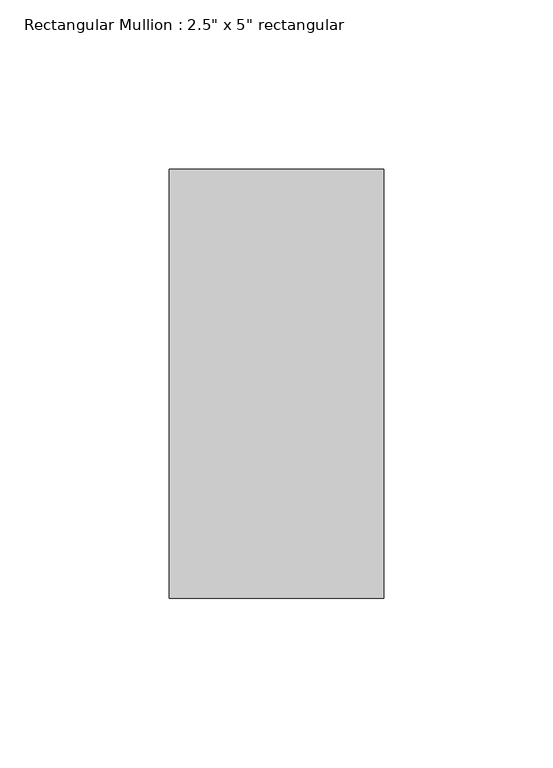
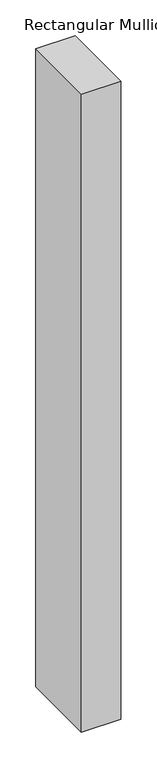
"""IFC4 building model written with IfcOpenShell, lengths in millimetres: member geometry."""

from ifc_helpers import new_model, si_unit, frame, origin, place, context, project, spatial, polyline, outline, extrude, source, transform, mapped, element, save


def member_95280835(model_context):
    return source(origin(), model_context, "Body", "SweptSolid", [
        extrude(outline(polyline([(0.0, 63.5), (0.0, -63.5), (-63.5, -63.5), (-63.5, 63.5), (0.0, 63.5)])), frame((0.0, 0.0, -1085.85), z_axis=(0.0, 0.0, 1.0), x_axis=(1.0, 0.0, 0.0)), (0.0, 0.0, 1.0), 1085.85),
    ])


if __name__ == "__main__":
    model = new_model("IFC4")
    model_context = context("Model", 3, world=origin())
    ifc_project = project(units=[si_unit("LENGTHUNIT", "METRE", prefix="MILLI")], contexts=[model_context])
    site = spatial("IfcSite", under=ifc_project)
    building = spatial("IfcBuilding", under=site)
    placement = place(None, origin())
    member_shape = member_95280835(model_context)
    element("IfcMember", 1, ObjectType="Rectangular Mullion : 2.5\" x 5\" rectangular", at=placement, inside=building, context=model_context, shape_type="MappedRepresentation", body=[
        mapped(member_shape, transform((0.0, 0.0, 0.0), x_axis=(1.0, 0.0, 0.0), y_axis=(0.0, 1.0, 0.0), z_axis=(0.0, 0.0, 1.0))),
    ])
    save(model, "model.ifc")

# Revit data of these elements
# Type "Rectangular Mullion : 2.5\" x 5\" rectangular"
#   built-in parameter 1007304 = 0.416667 (stored number, unit not read)
#   built-in parameter 1007301 = 0.104167 (stored number, unit not read)
#   built-in parameter 1007300 = 0.104167 (stored number, unit not read)
# Element 1 (IfcMember, "Rectangular Mullion : 2.5\" x 5\" rectangular")
#   Materials on its faces: "Aluminum"
# Materials
#   "Aluminum": class "Metal", colour RGB 247 247 247, transparency 0, Description = "Aluminum 6061", Cost = 0
